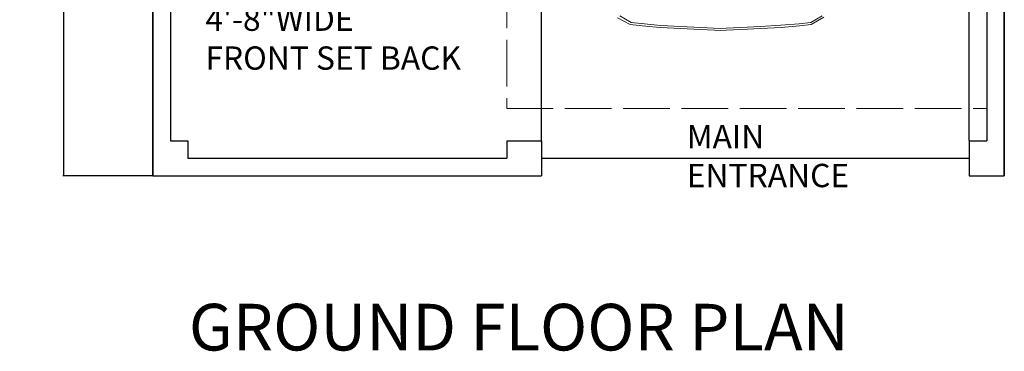
# Model space of a CAD drawing. Units: inches. Extents: x -16 to 587, y -783 to 64.
# Tile 1 of 14: x -16 to 237, y -783 to -697. Entities that reach past the tile are written whole.
import ezdxf

# ---------------------------------------------------------------- set-up
doc = ezdxf.new("R2010")
doc.units = ezdxf.units.IN
doc.header["$MEASUREMENT"] = 0
doc.linetypes.add('ACAD_ISO02W100', pattern=[15, 12, -3])
for name, color, linetype, lineweight in [('A-ANNO-DIMS', 2, 'Continuous', 18), ('A-ANNO-TEXT', 7, 'Continuous', 25), ('A-AREA-IDEN', 7, 'Continuous', 18), ('A-DOOR', 3, 'Continuous', 25), ('A-FLOR-OVHD', 8, 'ACAD_ISO02W100', 18), ('A-SITE-VEHC', 8, 'Continuous', 13), ('A-SITE-WALL', 7, 'Continuous', 30), ('A-WALL', 7, 'Continuous', 35)]:
    doc.layers.add(name, color=color, linetype=linetype, lineweight=lineweight)
doc.styles.get("Standard").update_dxf_attribs({"font": 'arial.ttf'})
doc.dimstyles.get("Standard").update_dxf_attribs({"dimtxt": 0.18, "dimasz": 0.18, "dimexe": 0.18, "dimexo": 0.0625, "dimgap": 0.09, "dimtad": 0, "dimtih": 1, "dimtoh": 1, "dimdec": 0, "dimzin": 0, "dimdsep": 46, "dimlunit": 3, "dimtxsty": 'Standard', "dimcen": 0.09, "dimadec": 0, "dimazin": 0, "dimtfac": 1, "dimtdec": 0, "dimtofl": 0, "dimtmove": 0, "dimatfit": 3, "dimfxl": 1, "dimtolj": 1, "dimtzin": 0, "dimarcsym": 0})

# ---------------------------------------------------------------- blocks, each defined once
blk = doc.blocks.new('*D6')
at = {"layer": 'A-ANNO-DIMS', "color": 0, "lineweight": -2, "transparency": 16777216}
for p, q in [((18.02, 19.45), (-5.05, 19.45)), ((-4.87, 19.27), (-4.87, -355.9)), ((-4.87, -737.37), (-4.87, -362.21)), ((18.02, -737.55), (-5.05, -737.55))]:
    blk.add_line(p, q, dxfattribs=at)
at = {"layer": 'A-ANNO-DIMS', "color": 0, "transparency": 16777216}
for points in [[(-4.9, 19.27), (-4.84, 19.27), (-4.87, 19.45)], [(-4.9, -737.37), (-4.84, -737.37), (-4.87, -737.55)]]:
    blk.add_solid(points, dxfattribs=at)
at = {"layer": 'Defpoints', "color": 0, "transparency": 16777216}
for p in [(18.08, 19.45), (-4.87, -737.55), (18.08, -737.55)]:
    blk.add_point(p, dxfattribs=at)
at = {"layer": 'A-ANNO-DIMS', "color": 0, "transparency": 16777216, "insert": (-4.87, -359.05), "char_height": 6, "attachment_point": 5}
blk.add_mtext('\\A1;63\'-1"', dxfattribs=at)
blk = doc.blocks.new('*D56')
at = {"layer": 'A-ANNO-DIMS', "color": 0, "lineweight": -2, "transparency": 16777216}
for p, q in [((118.08, -728.49), (118.08, 63.78)), ((118.26, 63.6), (172.75, 63.6)), ((227.9, 63.6), (173.41, 63.6)), ((228.08, -728.49), (228.08, 63.78))]:
    blk.add_line(p, q, dxfattribs=at)
at = {"layer": 'A-ANNO-DIMS', "color": 0, "transparency": 16777216}
for points in [[(118.26, 63.63), (118.26, 63.57), (118.08, 63.6)], [(227.9, 63.63), (227.9, 63.57), (228.08, 63.6)]]:
    blk.add_solid(points, dxfattribs=at)
at = {"layer": 'Defpoints', "color": 0, "transparency": 16777216}
for p in [(228.08, 63.6), (118.08, -728.55), (228.08, -728.55)]:
    blk.add_point(p, dxfattribs=at)
at = {"layer": 'A-ANNO-DIMS', "color": 0, "transparency": 16777216, "insert": (173.08, 63.6), "char_height": 0.18, "attachment_point": 5}
blk.add_mtext('\\A1;9\'-2"', dxfattribs=at)

msp = doc.modelspace()

# ---------------------------------------------------------------- linework, layer by layer
at = {"layer": 'A-DOOR'}
msp.add_line((118.08, -733.05), (228.08, -733.05), dxfattribs=at)
at = {"layer": 'A-FLOR-OVHD'}
for p, q in [((109.08, -672.55), (109.08, -720.26)), ((109.08, -720.26), (232.58, -720.26))]:
    msp.add_line(p, q, dxfattribs=at)
at = {"layer": 'A-SITE-VEHC'}
for p, q in [((138.17, -696.41), (141.09, -698.1)), ((187.34, -698.08), (190.25, -696.42)), ((140.84, -698.62), (137.62, -696.93)), ((143.91, -699), (140.84, -698.62)), ((141.09, -698.1), (148.74, -698.84)), ((148.58, -699.37), (143.91, -699)), ((148.74, -698.84), (158.93, -699.4)), ((174.36, -699.14), (179.64, -698.82)), ((179.64, -698.82), (184.29, -698.46)), ((184.38, -699), (179.71, -699.37)), ((184.29, -698.46), (187.34, -698.08)), ((187.44, -698.62), (184.38, -699)), ((190.62, -696.78), (187.44, -698.62)), ((153.89, -699.69), (148.58, -699.37)), ((158.87, -699.94), (153.89, -699.69)), ((162.57, -700.11), (158.87, -699.94)), ((158.93, -699.4), (164.03, -699.62)), ((164.01, -700.17), (162.57, -700.11)), ((165.52, -700.11), (164.01, -700.17)), ((164.03, -699.62), (165.53, -699.56)), ((169.34, -699.94), (165.52, -700.11)), ((165.53, -699.56), (169.33, -699.39)), ((169.33, -699.39), (174.36, -699.14)), ((174.39, -699.69), (169.34, -699.94)), ((179.71, -699.37), (174.39, -699.69))]:
    msp.add_line(p, q, dxfattribs=at)
at = {"layer": 'A-SITE-WALL'}
for p, q in [((232.58, -543.55), (232.58, -728.55)), ((22.58, -672.55), (22.58, -728.55)), ((22.58, -728.55), (27.08, -728.55)), ((27.08, -728.55), (27.08, -733.05)), ((109.08, -728.55), (109.08, -733.05)), ((109.08, -728.55), (118.08, -728.55)), ((118.08, -728.55), (118.08, -737.55)), ((228.08, -728.55), (232.58, -728.55)), ((228.08, -728.55), (228.08, -737.55)), ((27.08, -733.05), (109.08, -733.05)), ((18.08, -737.55), (118.08, -737.55)), ((228.08, -737.55), (237.08, -737.55))]:
    msp.add_line(p, q, dxfattribs=at)
at = {"layer": 'A-WALL'}
for p, q in [((18.08, 19.45), (18.08, -737.55)), ((237.08, 19.45), (237.08, -737.55))]:
    msp.add_line(p, q, dxfattribs=at)

# ---------------------------------------------------------------- texts
at = {"layer": 'A-ANNO-TEXT', "insert": (155.4, -724.47), "char_height": 6, "attachment_point": 1}
msp.add_mtext('MAIN\\PENTRANCE', dxfattribs=at)
at = {"layer": 'A-ANNO-TEXT', "insert": (27.34, -770.48), "char_height": 12, "width": 208.3399, "attachment_point": 1}
msp.add_mtext('GROUND FLOOR PLAN', dxfattribs=at)
at = {"layer": 'A-AREA-IDEN', "insert": (31.59, -694.26), "char_height": 6, "attachment_point": 1}
msp.add_mtext('4\'-8"WIDE\\PFRONT SET BACK', dxfattribs=at)

# ---------------------------------------------------------------- dimensions: what is measured, and where the dimension line sits
at = {"layer": 'A-ANNO-DIMS'}
dim = msp.add_linear_dim(base=(228.08, 63.6), p1=(118.08, -728.55), p2=(228.08, -728.55), dimstyle='Standard', override={"dimdec": 1, "dimlfac": 1, "dimrnd": 0, "dimzin": 1, "dimdsep": 46, "dimlunit": 4, "dimfrac": 2}, dxfattribs=at)
dim.commit()
dim.dimension.update_dxf_attribs({"geometry": '*D56', "text_midpoint": (173.08, 63.6)})
dim = msp.add_linear_dim(base=(-4.87, -737.55), p1=(18.08, 19.45), p2=(18.08, -737.55), angle=90, dimstyle='Standard', override={"dimtxt": 6, "dimclrd": 0, "dimclre": 0, "dimclrt": 0}, dxfattribs=at)
dim.commit()
dim.dimension.update_dxf_attribs({"geometry": '*D6', "text_midpoint": (-4.87, -359.05)})

doc.saveas('drawing.dxf')
